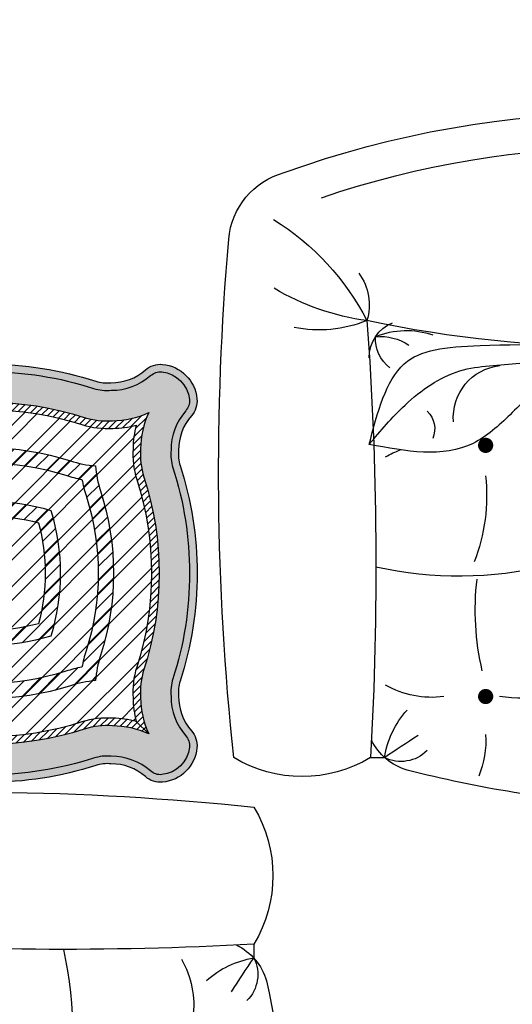
# Model space of a CAD drawing. Units: inches. Extents: x 844 to 2234, y 346 to 1084.
# Tile 23 of 93: x 1105 to 1116, y 710 to 731. Entities that reach past the tile are written whole.
import ezdxf

# ---------------------------------------------------------------- set-up
doc = ezdxf.new("R2010")
doc.units = ezdxf.units.IN
doc.header["$MEASUREMENT"] = 0
doc.layers.add('A-ANNO-DIMS', color=2, linetype='Continuous', lineweight=18)
doc.layers.add('furniture', color=8, linetype='Continuous', lineweight=18)
for name, color, linetype in [('RA-AP-01$0$FURN', 3, 'Continuous'), ('RA-AP-01$0$steel', 193, 'Continuous'), ('RA-AP-01$0$WOOD', 64, 'Continuous')]:
    doc.layers.add(name, color=color, linetype=linetype)
doc.styles.get("Standard").update_dxf_attribs({"font": 'arial.ttf'})
doc.dimstyles.get("Standard").update_dxf_attribs({"dimtxt": 6, "dimasz": 3, "dimexe": 0.18, "dimexo": 0.0625, "dimgap": 0.09, "dimtad": 0, "dimtih": 1, "dimtoh": 1, "dimdec": 1, "dimzin": 0, "dimdsep": 46, "dimlunit": 3, "dimtxsty": 'Standard', "dimblk": 'ARCHTICK', "dimcen": 0.09, "dimadec": 0, "dimazin": 0, "dimtfac": 1, "dimtdec": 1, "dimtofl": 0, "dimtmove": 0, "dimatfit": 3, "dimfxl": 1, "dimtolj": 1, "dimtzin": 0, "dimarcsym": 0})
pattern_1 = [(45, (0, 1.362436106329781), (-0.0088388347648318, 0.0088388347648318), [])]
pattern_2 = [(45, (0, 1.362436106329781), (-0.0044194173824159, 0.0044194173824159), [])]

# ---------------------------------------------------------------- blocks, each defined once
blk = doc.blocks.new('A$C2FCF5309')
at = {"layer": 'RA-AP-01$0$FURN'}
h = blk.add_hatch(dxfattribs=at)
h.set_pattern_fill('ANSI31', color=256, scale=0.1, style=0)
h.set_pattern_definition(pattern_1)
h.paths.add_polyline_path([(5.038683893313746, -5.169250834004607, -0.1583983521602212), (5.038683893312098, -5.373464580902012, 0.0306258898943267), (5.033304057242972, -5.394827569605182, 0.0306258898948892), (5.01194106853941, -5.40020740567441, -0.1028142994996694), (4.878286182323899, -5.414871334512708), (4.863600873530158, -5.43331743520547, 0.1120482678681049), (5.018059823131753, -5.419248541734471, -0.052642197802937), (5.050972078299936, -5.412495590662115, -0.0526421977994963), (5.057725029371615, -5.379583335496025, 0.1583028414702701), (5.057725029372958, -5.163132079409654, -0.052642197806903), (5.050972078299777, -5.130219824239078, -0.0526421977995126), (5.018059823133679, -5.123466873167369, 0.0215995840215353), (4.988903013548211, -5.115372132362452), (4.975007495303644, -5.132826183367946, -0.0289147572844802), (5.011941068537408, -5.142508009226167, 0.0306258898976746), (5.033304057242868, -5.147887845296027, 0.0306258899022411)])
h.paths.add_polyline_path([(4.975007495303645, -5.132826183367946), (4.988903013548211, -5.115372132362452, 0.1362374241599938), (4.801608567045604, -5.12346687316654, -0.0526421978036853), (4.768696311876971, -5.130219824239102, -0.05264219780204), (4.761943360804856, -5.163132079406747, 0.1583028414743723), (4.761943360806116, -5.379583335498449, -0.0526421977955461), (4.768696311877141, -5.412495590662114, -0.0526421978073986), (4.801608567048022, -5.419248541735437, 0.0454484293938888), (4.863600873530158, -5.43331743520547), (4.878286182323899, -5.414871334512708, -0.0546933379798044), (4.80772732164382, -5.40020740567649, 0.030625889903973), (4.786364332934043, -5.394827569605216, 0.0306258898932853), (4.780984496865101, -5.373464580902791, -0.1583983521638281), (4.780984496864308, -5.169250834000963, 0.03062588989692), (4.786364332933943, -5.147887845296004, 0.0306258898946324), (4.807727321637318, -5.142508009226805, -0.1288932573266927)])
h.paths.add_polyline_path([(4.843422214712861, -5.204945727074827, -0.0783685831716868), (4.924134454130224, -5.196727409635105), (4.939146578618322, -5.177870798323143, 0.1012675676854134), (4.827248748758957, -5.188772261120899, 0.1253648873081696), (4.820394258584192, -5.327034652050361), (4.837127701354095, -5.306015906404253, -0.0981593964869636)], flags=17)
h.paths.add_polyline_path([(4.843422214712824, -5.337769687826355, -0.0311091841722656), (4.837127701354095, -5.306015906404253), (4.820394258584193, -5.32703465205036, 0.0247727657431944), (4.827248748758908, -5.353943153780261, 0.0812754385032542), (4.916962478476905, -5.36629034358622), (4.933684093813825, -5.345286454285511, -0.0876255421014372)], flags=17)
h.paths.add_polyline_path([(4.992419641418037, -5.353943153780226, 0.1506053783834298), (4.992419641417933, -5.188772261120954, 0.0485966419124224), (4.939146578618321, -5.177870798323143), (4.924134454130224, -5.196727409635105, -0.0507799419579301), (4.976246175464031, -5.204945727074882, -0.1296645318906876), (4.97624617546411, -5.337769687826316, -0.0415667119298777), (4.933684093813825, -5.345286454285511), (4.916962478476905, -5.36629034358622, 0.0684915676023693)], flags=17)
h = blk.add_hatch(dxfattribs=at)
h.set_pattern_fill('ANSI31', color=256, scale=0.1, style=0)
h.set_pattern_definition(pattern_1)
h.paths.add_polyline_path([(5.038683893313746, -5.169250834004607, -0.1583983521602212), (5.038683893312098, -5.373464580902012, 0.0306258898943267), (5.033304057242972, -5.394827569605182, 0.0306258898948892), (5.01194106853941, -5.40020740567441, -0.1028142994996694), (4.878286182323899, -5.414871334512708), (4.863600873530158, -5.43331743520547, 0.1120482678681049), (5.018059823131753, -5.419248541734471, -0.052642197802937), (5.050972078299936, -5.412495590662115, -0.0526421977994963), (5.057725029371615, -5.379583335496025, 0.1583028414702701), (5.057725029372958, -5.163132079409654, -0.052642197806903), (5.050972078299777, -5.130219824239078, -0.0526421977995126), (5.018059823133679, -5.123466873167369, 0.0215995840215353), (4.988903013548211, -5.115372132362452), (4.975007495303644, -5.132826183367946, -0.0289147572844802), (5.011941068537408, -5.142508009226167, 0.0306258898976746), (5.033304057242868, -5.147887845296027, 0.0306258899022411)])
h.paths.add_polyline_path([(4.975007495303645, -5.132826183367946), (4.988903013548211, -5.115372132362452, 0.1362374241599938), (4.801608567045604, -5.12346687316654, -0.0526421978036853), (4.768696311876971, -5.130219824239102, -0.05264219780204), (4.761943360804856, -5.163132079406747, 0.1583028414743723), (4.761943360806116, -5.379583335498449, -0.0526421977955461), (4.768696311877141, -5.412495590662114, -0.0526421978073986), (4.801608567048022, -5.419248541735437, 0.0454484293938888), (4.863600873530158, -5.43331743520547), (4.878286182323899, -5.414871334512708, -0.0546933379798044), (4.80772732164382, -5.40020740567649, 0.030625889903973), (4.786364332934043, -5.394827569605216, 0.0306258898932853), (4.780984496865101, -5.373464580902791, -0.1583983521638281), (4.780984496864308, -5.169250834000963, 0.03062588989692), (4.786364332933943, -5.147887845296004, 0.0306258898946324), (4.807727321637318, -5.142508009226805, -0.1288932573266927)])
h.paths.add_polyline_path([(4.843422214712861, -5.204945727074827, -0.0783685831716868), (4.924134454130224, -5.196727409635105), (4.939146578618322, -5.177870798323143, 0.1012675676854134), (4.827248748758957, -5.188772261120899, 0.1253648873081696), (4.820394258584192, -5.327034652050361), (4.837127701354095, -5.306015906404253, -0.0981593964869636)], flags=17)
h.paths.add_polyline_path([(4.843422214712824, -5.337769687826355, -0.0311091841722656), (4.837127701354095, -5.306015906404253), (4.820394258584193, -5.32703465205036, 0.0247727657431944), (4.827248748758908, -5.353943153780261, 0.0812754385032542), (4.916962478476905, -5.36629034358622), (4.933684093813825, -5.345286454285511, -0.0876255421014372)], flags=17)
h.paths.add_polyline_path([(4.992419641418037, -5.353943153780226, 0.1506053783834298), (4.992419641417933, -5.188772261120954, 0.0485966419124224), (4.939146578618321, -5.177870798323143), (4.924134454130224, -5.196727409635105, -0.0507799419579301), (4.976246175464031, -5.204945727074882, -0.1296645318906876), (4.97624617546411, -5.337769687826316, -0.0415667119298777), (4.933684093813825, -5.345286454285511), (4.916962478476905, -5.36629034358622, 0.0684915676023693)], flags=17)
at = {"layer": 'RA-AP-01$0$WOOD'}
h = blk.add_hatch(color=256, dxfattribs=at)
edge = h.paths.add_edge_path()
edge.add_arc((4.683001772622394, -5.026441828662609), 0.0299999999999998, 48.77105092035535, 95.25687599427813)
edge.add_arc((4.684834195088484, -5.046357707450686), 0.0499999999998897, 95.25687599443106, 174.7431240064049)
edge.add_arc((4.664918316300367, -5.044525284985046), 0.0300000000000005, 174.7431240062535, 221.2289490796905)
edge.add_arc((4.591236830209155, -5.109094338216345), 0.0679700159630267, -0.5333070513215148, 41.228949079691915, ccw=False)
edge.add_arc((4.609451302807284, -5.114694777173187), 0.0500000000000008, -17.3556839752095, 5.7020707654044145, ccw=False)
edge.add_arc((5.095208119646659, -5.271357707450659), 0.4603971832811796, 162.0683908477609, 197.9316091523306)
edge.add_arc((4.609451302807533, -5.428020637728902), 0.0500000000000006, -5.702070765320514, 17.355683975293914, ccw=False)
edge.add_arc((4.591236830209412, -5.433621076685779), 0.0679700159630261, -41.228949079600625, 0.5333070514128053, ccw=False)
edge.add_arc((4.664918316300727, -5.498190129916959), 0.0299999999999995, 138.7710509204022, 185.256875994324)
edge.add_arc((4.684834195088642, -5.496357707450695), 0.0499999999997451, 185.2568759946742, 264.74312400432)
edge.add_arc((4.683001772622394, -5.516273586238612), 0.03, 264.743124003969, 311.2289490796446)
edge.add_arc((4.747570825853633, -5.589955072329876), 0.0679700159630271, 89.4666929486321, 131.2289490796457, ccw=False)
edge.add_arc((4.753171264810493, -5.57174059973175), 0.0500000000000015, 72.64431602474701, 95.70207076536133, ccw=False)
edge.add_arc((4.909834195088355, -5.085983782892503), 0.4603971832811774, 252.0683908477147, 287.9316091522845)
edge.add_arc((5.06649712536621, -5.57174059973175), 0.0499999999999999, 84.29792923463953, 107.35568397525361, ccw=False)
edge.add_arc((5.072097564323069, -5.589955072329877), 0.0679700159630274, 48.771050920354185, 90.5333070513679, ccw=False)
edge.add_arc((5.136666617554309, -5.516273586238614), 0.0299999999999997, 228.771050920353, 275.2568759942969)
edge.add_arc((5.134834195088338, -5.496357707450417), 0.0499999999999982, 275.2568759942949, 354.7431240057633)
edge.add_arc((5.154750073876535, -5.498190129916372), 0.0299999999999999, 354.7431240057662, 401.2289490796891)
edge.add_arc((5.228431559967749, -5.433621076685074), 0.0679700159630274, 179.4666929486771, 221.2289490796903, ccw=False)
edge.add_arc((5.210217087369615, -5.428020637728227), 0.0499999999999976, 162.6443160247947, 185.7020707654089, ccw=False)
edge.add_arc((4.724460270530244, -5.271357707450757), 0.4603971832811793, 342.0683908477607, 377.9316091523305)
edge.add_arc((5.210217087369368, -5.114694777172509), 0.0500000000000019, 174.2979292346878, 197.355683975302, ccw=False)
edge.add_arc((5.228431559967489, -5.109094338215639), 0.0679700159630279, 138.7710509203993, 180.5333070514128, ccw=False)
edge.add_arc((5.154750073876174, -5.044525284984457), 0.0300000000000001, 318.771050920401, 365.2568759954636)
edge.add_arc((5.13483419508816, -5.046357707450624), 0.0499999999998349, 5.256875995237118, 84.74312400549572)
edge.add_arc((5.136666617554308, -5.026441828662608), 0.0299999999999994, 84.74312400572185, 131.2289490796446)
edge.add_arc((5.072097564323072, -4.952760342571343), 0.0679700159630261, 269.4666929486298, 311.22894907964354, ccw=False)
edge.add_arc((5.066497125366206, -4.97097481516947), 0.0499999999999992, 252.64431602475162, 275.70207076536565, ccw=False)
edge.add_arc((4.909834195088355, -5.456731632008717), 0.4603971832811764, 72.06839084771546, 107.9316091522853)
edge.add_arc((4.753171264810493, -4.970974815169471), 0.0500000000000016, 264.2979292346387, 287.355683975253, ccw=False)
edge.add_arc((4.747570825853633, -4.952760342571346), 0.0679700159630274, 228.7710509203543, 270.5333070513679, ccw=False)
edge = h.paths.add_edge_path(flags=16)
edge.add_arc((4.683001772622395, -5.026441828662608), 0.019999999999999, 48.7710509203555, 95.2568759942793)
edge.add_arc((4.684834195088469, -5.046357707450671), 0.0399999999998731, 95.2568759944489, 174.7431240064248)
edge.add_arc((4.664918316300404, -5.044525284985035), 0.020000000000036, 174.7431240062186, 221.2289490796461)
edge.add_arc((4.591236830209151, -5.109094338216346), 0.0779700159630296, -0.13764630038667747, 41.228949079689585, ccw=False)
edge.add_arc((4.609451302807307, -5.11469477717304), 0.060000000000024, -17.406127045137907, 5.176192161068002, ccw=False)
edge.add_arc((5.09520811964665, -5.271357707450659), 0.4503971832811708, 162.0623235129628, 197.9376764869162)
edge.add_arc((4.609451302807532, -5.428020637728943), 0.0599999999999982, -5.176192160466428, 17.406127046715312, ccw=False)
edge.add_arc((4.591236830209414, -5.433621076685778), 0.0779700159630257, -41.2289490796029, 0.13764630095249686, ccw=False)
edge.add_arc((4.664918316300731, -5.498190129916961), 0.0200000000000047, 138.7710509204103, 185.2568759943212)
edge.add_arc((4.684834195088606, -5.496357707450731), 0.0399999999997066, 185.2568759947174, 264.7431240043665)
edge.add_arc((4.683001772622369, -5.516273586238541), 0.020000000000069, 264.7431240038842, 311.2289490795622)
edge.add_arc((4.747570825853635, -5.589955072329884), 0.0779700159630344, 89.8623536987642, 131.2289490796432, ccw=False)
edge.add_arc((4.753171264810603, -5.571740599731771), 0.0599999999999895, 72.5938729544394, 95.1761921602253, ccw=False)
edge.add_arc((4.909834195088365, -5.085983782892505), 0.4503971832811724, 252.0623235129989, 287.9376764870498)
edge.add_arc((5.066497125366216, -5.571740599731755), 0.0600000000000047, 84.8238078399923, 107.40612704528041, ccw=False)
edge.add_arc((5.072097564322998, -5.589955072329853), 0.077970015963056, 48.771050920303594, 90.13764630126451, ccw=False)
edge.add_arc((5.136666617554307, -5.516273586238622), 0.0199999999999931, 228.771050920344, 275.2568759943037)
edge.add_arc((5.134834195088338, -5.496357707450416), 0.0400000000000004, 275.2568759942928, 354.7431240057607)
edge.add_arc((5.154750073876533, -5.498190129916375), 0.0200000000000037, 354.7431240057783, 401.2289490796939)
edge.add_arc((5.228431559967745, -5.433621076685076), 0.0779700159630239, 179.8623536995147, 221.2289490796908, ccw=False)
edge.add_arc((5.210217087369586, -5.428020637728345), 0.0600000000000054, 162.5938729554486, 185.1761921609759, ccw=False)
edge.add_arc((4.724460270530243, -5.271357707450766), 0.4503971832811826, 342.0623235128896, 377.937676486982)
edge.add_arc((5.210217087369347, -5.114694777172486), 0.0599999999999777, 174.8238078387611, 197.4061270462219, ccw=False)
edge.add_arc((5.228431559967523, -5.109094338215542), 0.0779700159629885, 138.7710509204687, 180.1376463004423, ccw=False)
edge.add_arc((5.154750073876175, -5.044525284984459), 0.0199999999999989, 318.771050920406, 365.2568759954698)
edge.add_arc((5.134834195088138, -5.046357707450646), 0.0399999999998586, 5.256875995208452, 84.74312400546732)
edge.add_arc((5.136666617554292, -5.02644182866256), 0.0199999999999529, 84.74312400577769, 131.2289490797025)
edge.add_arc((5.072097564323069, -4.952760342571338), 0.077970015963032, 269.86235369901414, 311.2289490796421, ccw=False)
edge.add_arc((5.06649712536618, -4.97097481516946), 0.0600000000000007, 252.5938729548277, 275.17619216047467, ccw=False)
edge.add_arc((4.909834195088353, -5.456731632008716), 0.4503971832811739, 72.06232351293887, 107.9376764867365)
edge.add_arc((4.753171264810429, -4.970974815169467), 0.0599999999999991, 264.82380783985815, 287.40612704769893, ccw=False)
edge.add_arc((4.747570825853681, -4.952760342571361), 0.0779700159630467, 228.7710509203206, 270.13764630113724, ccw=False)
h = blk.add_hatch(color=256, dxfattribs=at)
edge = h.paths.add_edge_path()
edge.add_arc((4.683001772622395, -5.026441828662608), 0.019999999999999, 48.7710509203555, 95.2568759942793)
edge.add_arc((4.684834195088469, -5.046357707450671), 0.0399999999998731, 95.2568759944489, 174.7431240064248)
edge.add_arc((4.664918316300404, -5.044525284985035), 0.020000000000036, 174.7431240062186, 221.2289490796461)
edge.add_arc((4.591236830209151, -5.109094338216346), 0.0779700159630296, -0.13764630038667747, 41.228949079689585, ccw=False)
edge.add_arc((4.609451302807307, -5.11469477717304), 0.060000000000024, -17.406127045137907, 5.176192161068002, ccw=False)
edge.add_arc((5.09520811964665, -5.271357707450659), 0.4503971832811708, 162.0623235129628, 197.9376764869162)
edge.add_arc((4.609451302807532, -5.428020637728943), 0.0599999999999982, -5.176192160466428, 17.406127046715312, ccw=False)
edge.add_arc((4.591236830209414, -5.433621076685778), 0.0779700159630257, -41.2289490796029, 0.13764630095249686, ccw=False)
edge.add_arc((4.664918316300731, -5.498190129916961), 0.0200000000000047, 138.7710509204103, 185.2568759943212)
edge.add_arc((4.684834195088606, -5.496357707450731), 0.0399999999997066, 185.2568759947174, 264.7431240043665)
edge.add_arc((4.683001772622369, -5.516273586238541), 0.020000000000069, 264.7431240038842, 311.2289490795622)
edge.add_arc((4.747570825853635, -5.589955072329884), 0.0779700159630344, 89.8623536987642, 131.2289490796432, ccw=False)
edge.add_arc((4.753171264810603, -5.571740599731771), 0.0599999999999895, 72.5938729544394, 95.1761921602253, ccw=False)
edge.add_arc((4.909834195088365, -5.085983782892505), 0.4503971832811724, 252.0623235129989, 287.9376764870498)
edge.add_arc((5.066497125366216, -5.571740599731755), 0.0600000000000047, 84.8238078399923, 107.40612704528041, ccw=False)
edge.add_arc((5.072097564322998, -5.589955072329853), 0.077970015963056, 48.771050920303594, 90.13764630126451, ccw=False)
edge.add_arc((5.136666617554307, -5.516273586238622), 0.0199999999999931, 228.771050920344, 275.2568759943037)
edge.add_arc((5.134834195088338, -5.496357707450416), 0.0400000000000004, 275.2568759942928, 354.7431240057607)
edge.add_arc((5.154750073876533, -5.498190129916375), 0.0200000000000037, 354.7431240057783, 401.2289490796939)
edge.add_arc((5.228431559967745, -5.433621076685076), 0.0779700159630239, 179.8623536995147, 221.2289490796908, ccw=False)
edge.add_arc((5.210217087369586, -5.428020637728345), 0.0600000000000054, 162.5938729554486, 185.1761921609759, ccw=False)
edge.add_arc((4.724460270530243, -5.271357707450766), 0.4503971832811826, 342.0623235128896, 377.937676486982)
edge.add_arc((5.210217087369347, -5.114694777172486), 0.0599999999999777, 174.8238078387611, 197.4061270462219, ccw=False)
edge.add_arc((5.228431559967523, -5.109094338215542), 0.0779700159629885, 138.7710509204687, 180.1376463004423, ccw=False)
edge.add_arc((5.154750073876175, -5.044525284984459), 0.0199999999999989, 318.771050920406, 365.2568759954698)
edge.add_arc((5.134834195088138, -5.046357707450646), 0.0399999999998586, 5.256875995208452, 84.74312400546732)
edge.add_arc((5.136666617554292, -5.02644182866256), 0.0199999999999529, 84.74312400577769, 131.2289490797025)
edge.add_arc((5.072097564323069, -4.952760342571338), 0.077970015963032, 269.86235369901414, 311.2289490796421, ccw=False)
edge.add_arc((5.06649712536618, -4.97097481516946), 0.0600000000000007, 252.5938729548277, 275.17619216047467, ccw=False)
edge.add_arc((4.909834195088353, -5.456731632008716), 0.4503971832811739, 72.06232351293887, 107.9376764867365)
edge.add_arc((4.753171264810429, -4.970974815169467), 0.0599999999999991, 264.82380783985815, 287.40612704769893, ccw=False)
edge.add_arc((4.747570825853681, -4.952760342571361), 0.0779700159630467, 228.7710509203206, 270.13764630113724, ccw=False)
edge = h.paths.add_edge_path(flags=16)
edge.add_arc((4.591236830209151, -5.109094338216348), 0.1179700159630308, 0.7417751874182841, 24.563326950263672, ccw=False)
edge.add_arc((4.609451302807302, -5.114694777173093), 0.100000000000012, -17.52836504564658, 4.087328884225087, ccw=False)
edge.add_arc((5.095208119646651, -5.271357707450657), 0.4103971832811724, 162.0403002448777, 197.9596997550675)
edge.add_arc((4.60945130280753, -5.428020637728918), 0.1000000000000027, -4.087328883827581, 17.528365046291924, ccw=False)
edge.add_arc((4.591236830209414, -5.433621076685779), 0.1179700159630246, 335.43667305041845, 359.2582248129738, ccw=False)
edge.add_arc((4.747570825853596, -5.589955072329891), 0.117970015963042, 90.7417751868461, 114.5633269496104, ccw=False)
edge.add_arc((4.753171264810559, -5.571740599731767), 0.0999999999999976, 72.47163495370341, 94.0873288836737, ccw=False)
edge.add_arc((4.909834195088367, -5.085983782892503), 0.4103971832811735, 252.0403002449999, 287.9596997551833)
edge.add_arc((5.066497125366205, -5.571740599731755), 0.1000000000000057, 85.91267111645209, 107.5283650455624, ccw=False)
edge.add_arc((5.072097564322985, -5.58995507232986), 0.117970015963046, 65.4366730497672, 89.25822481317113, ccw=False)
edge.add_arc((5.22843155996773, -5.433621076684992), 0.1179700159630096, 180.7417751873964, 204.5633269502712, ccw=False)
edge.add_arc((5.210217087369591, -5.428020637728301), 0.0999999999999969, 162.4716349546276, 184.0873288841682, ccw=False)
edge.add_arc((4.724460270530243, -5.271357707450766), 0.4103971832811825, 342.0403002448147, 377.9596997550345)
edge.add_arc((5.210217087369347, -5.114694777172489), 0.0999999999999796, 175.9126711156995, 197.5283650464392, ccw=False)
edge.add_arc((5.228431559967512, -5.109094338215525), 0.1179700159630019, 155.4366730502992, 179.2582248126247, ccw=False)
edge.add_arc((5.072097564323172, -4.952760342571314), 0.1179700159630537, 270.74177518697286, 294.56332694975765, ccw=False)
edge.add_arc((5.066497125366189, -4.970974815169462), 0.1000000000000017, 252.471634954247, 274.0873288838353, ccw=False)
edge.add_arc((4.909834195088353, -5.456731632008716), 0.4103971832811758, 72.04030024486342, 107.9596997549354)
edge.add_arc((4.75317126481046, -4.970974815169467), 0.1000000000000041, 265.91267111635307, 287.5283650466103, ccw=False)
edge.add_arc((4.747570825853629, -4.952760342571342), 0.1179700159630538, 245.43667304992562, 269.2582248131125, ccw=False)
h = blk.add_hatch(dxfattribs=at)
h.set_pattern_fill('ANSI31', color=256, scale=0.05, style=0)
h.set_pattern_definition(pattern_2)
h.paths.add_polyline_path([(5.105336294329346, -5.394854099602528, 0.0940138826956367), (5.100476366643778, -5.435568764288975, 0.0606271852326483), (5.104678567100611, -5.466202079462671, 0.0606271852344644), (5.074045251925975, -5.46199987900586, 0.0940138827021426), (5.033330587236848, -5.466859806692645, -0.1305325492494615), (4.828072633169377, -5.477944178050054), (4.821119726105699, -5.486677669841435, 0.1336226599878005), (5.036379334063467, -5.476383803188216, -0.0945969211935747), (5.073624810952389, -5.471994942692536, -0.1043170707892296), (5.121137550891356, -5.48266106325342, -0.1043170707868944), (5.110471430330457, -5.435148323315565, -0.0945969211952573), (5.114860290825935, -5.397902846425963, 0.1580239521433527), (5.114860290826324, -5.144812568476775, -0.0945969212010491), (5.110471430330247, -5.10756709158498, -0.1043170707844371), (5.121137550890657, -5.060054351648168, -0.104317070786514), (5.073624810952866, -5.070720472208642, -0.0945969211958523), (5.036379334063063, -5.066331611712874, 0.1580239521426795), (4.783289056114906, -5.066331611712465, -0.0945969211985319), (4.746043579224103, -5.070720472208672, -0.1043170707882665), (4.698530839285552, -5.060054351647925, -0.1043170707867205), (4.709196959846443, -5.10756709158571, -0.094596921196788), (4.704808099350826, -5.144812568475902, 0.1580239521433127), (4.704808099350699, -5.397902846425022, -0.094596921197841), (4.709196959846712, -5.435148323315576, -0.1043170707855109), (4.698530839286393, -5.482661063252921, -0.1043170707864168), (4.746043579224162, -5.471994942692571, -0.0945969211977586), (4.783289056114671, -5.476383803188671, 0.0238966994662183), (4.821119726105699, -5.486677669841435), (4.828072633169378, -5.477944178050054, -0.0269814195959459), (4.786337802940177, -5.466859806692736, 0.0940138827039629), (4.745623138250268, -5.461999879005895, 0.0606271852320776), (4.714989823076826, -5.466202079462476, 0.0606271852304618), (4.719192023533341, -5.435568764289856, 0.0940138826917763), (4.714332095848404, -5.394854099604977, -0.1580706864542086), (4.714332095846561, -5.147861315302034, 0.0940138827032017), (4.719192023533127, -5.107146650612438, 0.0606271852329446), (4.714989823076289, -5.076513335438588, 0.0606271852340035), (4.745623138250698, -5.08071553589536, 0.0940138827025969), (4.786337802940015, -5.075855608208526, -0.1580706864508517), (5.033330587237968, -5.075855608208939, 0.0940138827009578), (5.074045251926627, -5.080715535895319, 0.0606271852322557), (5.104678567100159, -5.076513335438697, 0.0606271852308743), (5.100476366643561, -5.107146650611519, 0.0940138827178109), (5.105336294331983, -5.147861315307182, -0.1580706864490946)])
h = blk.add_hatch(dxfattribs=at)
h.set_pattern_fill('ANSI31', color=256, scale=0.05, style=0)
h.set_pattern_definition(pattern_2)
h.paths.add_polyline_path([(5.105336294329346, -5.394854099602528, 0.0940138826956367), (5.100476366643778, -5.435568764288975, 0.0606271852326483), (5.104678567100611, -5.466202079462671, 0.0606271852344644), (5.074045251925975, -5.46199987900586, 0.0940138827021426), (5.033330587236848, -5.466859806692645, -0.1305325492494615), (4.828072633169377, -5.477944178050054), (4.821119726105699, -5.486677669841435, 0.1336226599878005), (5.036379334063467, -5.476383803188216, -0.0945969211935747), (5.073624810952389, -5.471994942692536, -0.1043170707892296), (5.121137550891356, -5.48266106325342, -0.1043170707868944), (5.110471430330457, -5.435148323315565, -0.0945969211952573), (5.114860290825935, -5.397902846425963, 0.1580239521433527), (5.114860290826324, -5.144812568476775, -0.0945969212010491), (5.110471430330247, -5.10756709158498, -0.1043170707844371), (5.121137550890657, -5.060054351648168, -0.104317070786514), (5.073624810952866, -5.070720472208642, -0.0945969211958523), (5.036379334063063, -5.066331611712874, 0.1580239521426795), (4.783289056114906, -5.066331611712465, -0.0945969211985319), (4.746043579224103, -5.070720472208672, -0.1043170707882665), (4.698530839285552, -5.060054351647925, -0.1043170707867205), (4.709196959846443, -5.10756709158571, -0.094596921196788), (4.704808099350826, -5.144812568475902, 0.1580239521433127), (4.704808099350699, -5.397902846425022, -0.094596921197841), (4.709196959846712, -5.435148323315576, -0.1043170707855109), (4.698530839286393, -5.482661063252921, -0.1043170707864168), (4.746043579224162, -5.471994942692571, -0.0945969211977586), (4.783289056114671, -5.476383803188671, 0.0238966994662183), (4.821119726105699, -5.486677669841435), (4.828072633169378, -5.477944178050054, -0.0269814195959459), (4.786337802940177, -5.466859806692736, 0.0940138827039629), (4.745623138250268, -5.461999879005895, 0.0606271852320776), (4.714989823076826, -5.466202079462476, 0.0606271852304618), (4.719192023533341, -5.435568764289856, 0.0940138826917763), (4.714332095848404, -5.394854099604977, -0.1580706864542086), (4.714332095846561, -5.147861315302034, 0.0940138827032017), (4.719192023533127, -5.107146650612438, 0.0606271852329446), (4.714989823076289, -5.076513335438588, 0.0606271852340035), (4.745623138250698, -5.08071553589536, 0.0940138827025969), (4.786337802940015, -5.075855608208526, -0.1580706864508517), (5.033330587237968, -5.075855608208939, 0.0940138827009578), (5.074045251926627, -5.080715535895319, 0.0606271852322557), (5.104678567100159, -5.076513335438697, 0.0606271852308743), (5.100476366643561, -5.107146650611519, 0.0940138827178109), (5.105336294331983, -5.147861315307182, -0.1580706864490946)])
h = blk.add_hatch(dxfattribs=at)
h.set_pattern_fill('ANSI32,_I', color=256, scale=0.1, style=2)
h.set_pattern_definition([(45, (0, 0), (-0.0265165042944955, 0.0265165042944955), []), (45, (0.0176776695, 0), (-0.0265165042944955, 0.0265165042944955), [])])
h.paths.add_polyline_path([(4.843422214712824, -5.337769687826354, 0.1296645318905289), (4.97624617546411, -5.337769687826316, 0.1296645318906876), (4.976246175464032, -5.204945727074882, 0.129664531890418), (4.843422214712861, -5.204945727074827, 0.129664531890765)], flags=0)
h.paths.add_polyline_path([(5.039131224122924, -5.170637849998464, -0.0326520429852175), (5.033304057242868, -5.147887845296027, -0.0326520429894721), (5.010554052537512, -5.142060678415043, 0.1561383235202698), (4.809114337641437, -5.142060678414318, -0.0326520429925972), (4.786364332933944, -5.147887845296004, -0.0326520429914489), (4.780537166052582, -5.170637850002729, 0.1561383235189577), (4.780537166052134, -5.37207756489719, -0.0326520429934175), (4.786364332934042, -5.394827569605215, -0.0326520429823496), (4.809114337634529, -5.400654736484653, 0.156138323524066), (5.010554052535268, -5.400654736486903, -0.032652042992888), (5.033304057242972, -5.394827569605183, -0.0326520429928733), (5.039131224124712, -5.372077564897496, 0.1561383235226786)], flags=0)
h.paths.add_polyline_path([(4.992419641418037, -5.353943153780226, -0.1506053783832862), (4.827248748758909, -5.353943153780261, -0.1506053783835069), (4.827248748758957, -5.188772261120899, -0.1506053783831346), (4.992419641417933, -5.188772261120954, -0.1506053783834298)], flags=0)
h.paths.add_polyline_path([(4.976246175464111, -5.337769687826316, -0.1296645318905298), (4.843422214712824, -5.337769687826354, -0.129664531890765), (4.843422214712862, -5.204945727074827, -0.1296645318904162), (4.976246175464031, -5.204945727074882, -0.1296645318906876)], flags=0)
h.paths.add_polyline_path([(5.105721254232479, -5.149054940982025, -0.0968902512052664), (5.100476366643561, -5.107146650611519, -0.0606271852308743), (5.104678567100159, -5.076513335438697, -0.0606271852322574), (5.074045251926626, -5.080715535895319, -0.0968902512197216), (5.032136961550132, -5.075470648304253, 0.1564657949319774), (4.787531428625239, -5.075470648304682, -0.0968902512150626), (4.745623138250699, -5.08071553589536, -0.060627185234009), (4.714989823076288, -5.076513335438587, -0.0606271852329501), (4.719192023533127, -5.10714665061244, -0.0968902512185585), (4.713947135942331, -5.149054940988458, 0.1564657949285579), (4.713947135940853, -5.393660473908259, -0.0968902512319826), (4.71919202353334, -5.435568764289873, -0.0606271852304288), (4.714989823076825, -5.466202079462476, -0.0606271852320811), (4.745623138250269, -5.461999879005895, -0.0968902512162649), (4.787531428625332, -5.467244766596559, 0.1564657949327057), (5.032136961551311, -5.46724476659659, -0.0968902512153659), (5.074045251925975, -5.46199987900586, -0.0606271852344627), (5.10467856710061, -5.466202079462671, -0.0606271852326483), (5.100476366643777, -5.435568764288975, -0.0968902512258216), (5.105721254235559, -5.393660473909953, 0.1564657949340142)])
h.paths.add_polyline_path([(5.057725029371625, -5.379583335495999, 0.0526421977995391), (5.050972078299936, -5.412495590662114, 0.0526421978029782), (5.018059823131728, -5.419248541734479, -0.1583028414681072), (4.801608567048168, -5.419248541735485, 0.0526421978076402), (4.76869631187714, -5.412495590662113, 0.0526421977956189), (4.761943360806101, -5.379583335498404, -0.1583028414743129), (4.761943360804846, -5.163132079406778, 0.0526421978020944), (4.768696311876972, -5.130219824239101, 0.0526421978033651), (4.80160856704541, -5.123466873166602, -0.1583028414716875), (5.018059823133628, -5.123466873167353, 0.0526421977995944), (5.050972078299776, -5.130219824239078, 0.0526421978070423), (5.057725029372986, -5.163132079409739, -0.1583028414701848)], flags=16)
h.paths.add_polyline_path([(5.038683893312112, -5.373464580901968, 0.0306258898943915), (5.033304057242972, -5.394827569605182, 0.0306258898948892), (5.01194106853941, -5.40020740567441, -0.1583983521587032), (4.807727321643864, -5.400207405676503, 0.0306258899040366), (4.786364332934043, -5.394827569605215, 0.0306258898931986), (4.780984496865119, -5.37346458090285, -0.1583983521638542), (4.7809844968643, -5.169250834000989, 0.0306258898969596), (4.786364332933945, -5.147887845296004, 0.0306258898946195), (4.807727321637311, -5.142508009226808, -0.1583983521623412), (5.011941068537318, -5.142508009226139, 0.030625889897807), (5.033304057242868, -5.147887845296028, 0.0306258899020632), (5.038683893313706, -5.169250834004486, -0.1583983521602835)], flags=0)
for p, q in [((4.714989823076289, -5.076513335438588), (4.698530839285552, -5.060054351647925)), ((4.714989823076289, -5.076513335438588), (4.698530839285552, -5.060054351647925)), ((5.104678567100159, -5.076513335438697), (5.121137550890656, -5.060054351648169)), ((5.104678567100159, -5.076513335438697), (5.121137550890656, -5.060054351648169)), ((5.10467856710061, -5.466202079462671), (5.121137550891355, -5.482661063253419)), ((5.10467856710061, -5.466202079462671), (5.121137550891355, -5.482661063253419))]:
    blk.add_line(p, q, dxfattribs=at)
for points in [[(4.702773858784635, -5.003879368495489, 0.2056608120285223), (4.680253138923443, -4.996568010480312, 0.3614336704708569), (4.635044498118043, -5.041776651286372, 0.2056608120263112), (4.642355856133262, -5.064297371147306, -0.1842662638101064), (4.65920390179375, -5.10972699154053, -0.1009492694051416), (4.657174869772992, -5.129609908955028, 0.1577727036674954), (4.657174869773219, -5.41310550594699, -0.1009492694051416), (4.659203901794006, -5.432988423361486, -0.1842662638101064), (4.64235585613359, -5.478418043754737, 0.2056608120285221), (4.635044498118431, -5.500938763615934, 0.3614336704593693), (4.680253138922529, -5.546147404420826, 0.2056608120364936), (4.702773858784635, -5.538836046405732, -0.1842662638101064), (4.748203479177874, -5.52198800074528, -0.1009492694051415), (4.768086396592371, -5.524017032766053, 0.1577727036674954), (5.051581993584332, -5.524017032766055, -0.1009492694051416), (5.071464910998829, -5.521988000745282, -0.1842662638101064), (5.116894531392067, -5.538836046405734, 0.2056608120286145), (5.13941525125327, -5.546147404420911, 0.3614336704683636), (5.184623892058835, -5.500938763615299, 0.2056608120285223), (5.177312534043641, -5.478418043754112, -0.1842662638101063), (5.160464488383153, -5.432988423360887, -0.1009492694051416), (5.162493520403909, -5.41310550594639, 0.1577727036674954), (5.162493520403684, -5.129609908954428, -0.1009492694051416), (5.160464488382894, -5.109726991539933, -0.1842662638101064), (5.17731253404331, -5.064297371146681, 0.2056608120337072), (5.184623892058415, -5.041776651284888, 0.3614336704623863), (5.139415251253259, -4.99656801048031, 0.2056608120285223), (5.116894531392067, -5.003879368495487, -0.1842662638101064), (5.071464910998829, -5.020727414155937, -0.1009492694051416), (5.051581993584332, -5.018698382135166, 0.1577727036674956), (4.768086396592371, -5.018698382135168, -0.1009492694051416), (4.748203479177874, -5.020727414155941, -0.1842662638101064)], [(4.702773858784635, -5.003879368495489, 0.2056608120285223), (4.680253138923443, -4.996568010480312, 0.3614336704708569), (4.635044498118043, -5.041776651286372, 0.2056608120263112), (4.642355856133262, -5.064297371147306, -0.1842662638101064), (4.65920390179375, -5.10972699154053, -0.1009492694051416), (4.657174869772992, -5.129609908955028, 0.1577727036674954), (4.657174869773219, -5.41310550594699, -0.1009492694051416), (4.659203901794006, -5.432988423361486, -0.1842662638101064), (4.64235585613359, -5.478418043754737, 0.2056608120285221), (4.635044498118431, -5.500938763615934, 0.3614336704593693), (4.680253138922529, -5.546147404420826, 0.2056608120364936), (4.702773858784635, -5.538836046405732, -0.1842662638101064), (4.748203479177874, -5.52198800074528, -0.1009492694051415), (4.768086396592371, -5.524017032766053, 0.1577727036674954), (5.051581993584332, -5.524017032766055, -0.1009492694051416), (5.071464910998829, -5.521988000745282, -0.1842662638101064), (5.116894531392067, -5.538836046405734, 0.2056608120286145), (5.13941525125327, -5.546147404420911, 0.3614336704683636), (5.184623892058835, -5.500938763615299, 0.2056608120285223), (5.177312534043641, -5.478418043754112, -0.1842662638101063), (5.160464488383153, -5.432988423360887, -0.1009492694051416), (5.162493520403909, -5.41310550594639, 0.1577727036674954), (5.162493520403684, -5.129609908954428, -0.1009492694051416), (5.160464488382894, -5.109726991539933, -0.1842662638101064), (5.17731253404331, -5.064297371146681, 0.2056608120337072), (5.184623892058415, -5.041776651284888, 0.3614336704623863), (5.139415251253259, -4.99656801048031, 0.2056608120285223), (5.116894531392067, -5.003879368495487, -0.1842662638101064), (5.071464910998829, -5.020727414155937, -0.1009492694051416), (5.051581993584332, -5.018698382135166, 0.1577727036674956), (4.768086396592371, -5.018698382135168, -0.1009492694051416), (4.748203479177874, -5.020727414155941, -0.1842662638101064)], [(4.696183163397222, -5.011400188551196, 0.2056608120285295), (4.681169350156427, -5.006525949874411, 0.3614336704708588), (4.645002437512154, -5.042692862519237, 0.2056608120262659), (4.649876676188964, -5.057706675759887, -0.182481815856965), (4.669206621172843, -5.109281651732388, -0.0988540857970112), (4.666703803477437, -5.13264334722805, 0.1578269695851905), (4.666703803477144, -5.410072067672365, -0.0988540858013112), (4.6692066211731, -5.433433763168966, -0.1824818158591246), (4.649876676189301, -5.485008739142145, 0.2056608120284717), (4.64500243751253, -5.500022552382944, 0.3614336704593821), (4.681169350155757, -5.536189465026749, 0.2056608120365057), (4.696183163397221, -5.531315226350026, -0.1824818158605826), (4.747758139370833, -5.51198528136619, -0.0988540857951607), (4.771119834866025, -5.514488099061806, 0.1578269695856264), (5.04854855531107, -5.514488099061688, -0.0988540857929677), (5.071910250805761, -5.511985281366138, -0.1824818158609529), (5.123485226779481, -5.531315226350027, 0.2056608120286893), (5.138499040020282, -5.536189465026812, 0.3614336704683556), (5.174665952664737, -5.500022552382323, 0.2056608120284882), (5.169791713987938, -5.485008739141532, -0.1824818158574124), (5.150461769004059, -5.4334337631689, -0.0988540857940221), (5.152964586699289, -5.410072067673927, 0.1578269695858123), (5.1529645866996, -5.132643347228565, -0.0988540858025403), (5.150461769003872, -5.109281651731659, -0.1824818158565006), (5.169791713987599, -5.057706675759273, 0.2056608120337192), (5.174665952664335, -5.042692862518078, 0.3614336704623903), (5.138499040020236, -5.006525949874406, 0.2056608120285323), (5.123485226779481, -5.011400188551195, -0.1824818158594503), (5.071910250806212, -5.03073013353503, -0.09885408579455), (5.048548555311143, -5.028227315839558, 0.1578269695844942), (4.771119834867991, -5.028227315838772, -0.0988540858042156), (4.747758139370745, -5.030730133535067, -0.1824818158603032)], [(4.696183163397222, -5.011400188551196, 0.2056608120285295), (4.681169350156427, -5.006525949874411, 0.3614336704708588), (4.645002437512154, -5.042692862519237, 0.2056608120262659), (4.649876676188964, -5.057706675759887, -0.182481815856965), (4.669206621172843, -5.109281651732388, -0.0988540857970112), (4.666703803477437, -5.13264334722805, 0.1578269695851905), (4.666703803477144, -5.410072067672365, -0.0988540858013112), (4.6692066211731, -5.433433763168966, -0.1824818158591246), (4.649876676189301, -5.485008739142145, 0.2056608120284717), (4.64500243751253, -5.500022552382944, 0.3614336704593821), (4.681169350155757, -5.536189465026749, 0.2056608120365057), (4.696183163397221, -5.531315226350026, -0.1824818158605826), (4.747758139370833, -5.51198528136619, -0.0988540857951607), (4.771119834866025, -5.514488099061806, 0.1578269695856264), (5.04854855531107, -5.514488099061688, -0.0988540857929677), (5.071910250805761, -5.511985281366138, -0.1824818158609529), (5.123485226779481, -5.531315226350027, 0.2056608120286893), (5.138499040020282, -5.536189465026812, 0.3614336704683556), (5.174665952664737, -5.500022552382323, 0.2056608120284882), (5.169791713987938, -5.485008739141532, -0.1824818158574124), (5.150461769004059, -5.4334337631689, -0.0988540857940221), (5.152964586699289, -5.410072067673927, 0.1578269695858123), (5.1529645866996, -5.132643347228565, -0.0988540858025403), (5.150461769003872, -5.109281651731659, -0.1824818158565006), (5.169791713987599, -5.057706675759273, 0.2056608120337192), (5.174665952664335, -5.042692862518078, 0.3614336704623903), (5.138499040020236, -5.006525949874406, 0.2056608120285323), (5.123485226779481, -5.011400188551195, -0.1824818158594503), (5.071910250806212, -5.03073013353503, -0.09885408579455), (5.048548555311143, -5.028227315839558, 0.1578269695844942), (4.771119834867991, -5.028227315838772, -0.0988540858042156), (4.747758139370745, -5.030730133535067, -0.1824818158603032)], [(4.698530839285552, -5.060054351647925, -0.1043170707867612), (4.709196959846444, -5.107567091585729, -0.0945969211969405), (4.704808099350802, -5.144812568475978, 0.1580239521432241), (4.704808099350681, -5.397902846424963, -0.0945969211980322), (4.709196959846711, -5.43514832331559, -0.104317070785482), (4.698530839286393, -5.482661063252921, -0.1043170707864036), (4.746043579224155, -5.471994942692571, -0.094596921197375), (4.78328905611452, -5.476383803188623, 0.1580239521431959), (5.036379334063463, -5.476383803188218, -0.0945969211935888), (5.07362481095239, -5.471994942692536, -0.1043170707892253), (5.121137550891355, -5.482661063253419, -0.1043170707868921), (5.110471430330457, -5.435148323315565, -0.0945969211954828), (5.114860290825962, -5.397902846425878, 0.158023952143358), (5.114860290826295, -5.144812568476682, -0.0945969212007617), (5.110471430330247, -5.107567091584995, -0.1043170707844689), (5.121137550890656, -5.060054351648169, -0.1043170707864946), (5.073624810952874, -5.070720472208642, -0.0945969211956941), (5.036379334063131, -5.066331611712896, 0.1580239521426976), (4.783289056114946, -5.066331611712452, -0.0945969211986379), (4.746043579224103, -5.070720472208672, -0.1043170707882684)], [(4.698530839285552, -5.060054351647925, -0.1043170707867612), (4.709196959846444, -5.107567091585729, -0.0945969211969405), (4.704808099350802, -5.144812568475978, 0.1580239521432241), (4.704808099350681, -5.397902846424963, -0.0945969211980322), (4.709196959846711, -5.43514832331559, -0.104317070785482), (4.698530839286393, -5.482661063252921, -0.1043170707864036), (4.746043579224155, -5.471994942692571, -0.094596921197375), (4.78328905611452, -5.476383803188623, 0.1580239521431959), (5.036379334063463, -5.476383803188218, -0.0945969211935888), (5.07362481095239, -5.471994942692536, -0.1043170707892253), (5.121137550891355, -5.482661063253419, -0.1043170707868921), (5.110471430330457, -5.435148323315565, -0.0945969211954828), (5.114860290825962, -5.397902846425878, 0.158023952143358), (5.114860290826295, -5.144812568476682, -0.0945969212007617), (5.110471430330247, -5.107567091584995, -0.1043170707844689), (5.121137550890656, -5.060054351648169, -0.1043170707864946), (5.073624810952874, -5.070720472208642, -0.0945969211956941), (5.036379334063131, -5.066331611712896, 0.1580239521426976), (4.783289056114946, -5.066331611712452, -0.0945969211986379), (4.746043579224103, -5.070720472208672, -0.1043170707882684)], [(4.714989823076289, -5.076513335438588, -0.0606271852329464), (4.719192023533127, -5.107146650612439, -0.0940138827030756), (4.714332095846578, -5.147861315301983, 0.1580706864542707), (4.714332095848417, -5.394854099605018, -0.0940138826916965), (4.719192023533341, -5.435568764289864, -0.0606271852304462), (4.714989823076826, -5.466202079462476, -0.0606271852320585), (4.745623138250258, -5.461999879005895, -0.0940138827037036), (4.786337802940059, -5.466859806692699, 0.1580706864500221), (5.033330587236783, -5.466859806692666, -0.0940138827023111), (5.074045251925979, -5.46199987900586, -0.060627185234454), (5.10467856710061, -5.466202079462671, -0.0606271852326709), (5.100476366643777, -5.435568764288963, -0.0940138826958686), (5.105336294329379, -5.394854099602421, 0.1580706864489859), (5.105336294331999, -5.147861315307237, -0.0940138827179432), (5.100476366643561, -5.107146650611518, -0.0606271852308726), (5.104678567100159, -5.076513335438697, -0.0606271852322592), (5.074045251926625, -5.080715535895319, -0.094013882701022), (5.03333058723794, -5.075855608208931, 0.1580706864508015), (4.786337802940061, -5.075855608208511, -0.0940138827027143), (4.745623138250695, -5.08071553589536, -0.0606271852339983)], [(4.714989823076289, -5.076513335438588, -0.0606271852329464), (4.719192023533127, -5.107146650612439, -0.0940138827030756), (4.714332095846578, -5.147861315301983, 0.1580706864542707), (4.714332095848417, -5.394854099605018, -0.0940138826916965), (4.719192023533341, -5.435568764289864, -0.0606271852304462), (4.714989823076826, -5.466202079462476, -0.0606271852320585), (4.745623138250258, -5.461999879005895, -0.0940138827037036), (4.786337802940059, -5.466859806692699, 0.1580706864500221), (5.033330587236783, -5.466859806692666, -0.0940138827023111), (5.074045251925979, -5.46199987900586, -0.060627185234454), (5.10467856710061, -5.466202079462671, -0.0606271852326709), (5.100476366643777, -5.435568764288963, -0.0940138826958686), (5.105336294329379, -5.394854099602421, 0.1580706864489859), (5.105336294331999, -5.147861315307237, -0.0940138827179432), (5.100476366643561, -5.107146650611518, -0.0606271852308726), (5.104678567100159, -5.076513335438697, -0.0606271852322592), (5.074045251926625, -5.080715535895319, -0.094013882701022), (5.03333058723794, -5.075855608208931, 0.1580706864508015), (4.786337802940061, -5.075855608208511, -0.0940138827027143), (4.745623138250695, -5.08071553589536, -0.0606271852339983)], [(4.768696311876972, -5.130219824239102, -0.0526421978019087), (4.761943360804882, -5.163132079406667, 0.1583028414744761), (4.761943360806133, -5.379583335498504, -0.0526421977954539), (4.76869631187714, -5.412495590662113, -0.0526421978076619), (4.801608567048181, -5.419248541735488, 0.1583028414681522), (5.0180598231318, -5.419248541734456, -0.0526421978028585), (5.050972078299936, -5.412495590662114, -0.0526421977992923), (5.057725029371576, -5.379583335496149, 0.1583028414703719), (5.057725029372956, -5.163132079409646, -0.0526421978068888), (5.050972078299776, -5.130219824239078, -0.052642197799403), (5.018059823133745, -5.12346687316739, 0.1583028414717216), (4.801608567045482, -5.123466873166579, -0.0526421978034837)], [(4.768696311876972, -5.130219824239102, -0.0526421978019087), (4.761943360804882, -5.163132079406667, 0.1583028414744761), (4.761943360806133, -5.379583335498504, -0.0526421977954539), (4.76869631187714, -5.412495590662113, -0.0526421978076619), (4.801608567048181, -5.419248541735488, 0.1583028414681522), (5.0180598231318, -5.419248541734456, -0.0526421978028585), (5.050972078299936, -5.412495590662114, -0.0526421977992923), (5.057725029371576, -5.379583335496149, 0.1583028414703719), (5.057725029372956, -5.163132079409646, -0.0526421978068888), (5.050972078299776, -5.130219824239078, -0.052642197799403), (5.018059823133745, -5.12346687316739, 0.1583028414717216), (4.801608567045482, -5.123466873166579, -0.0526421978034837)], [(4.786364332933944, -5.147887845296004, -0.0306258898969254), (4.780984496864308, -5.169250834000966, 0.1583983521638412), (4.780984496865107, -5.373464580902811, -0.0306258898932568), (4.786364332934043, -5.394827569605216, -0.0306258899041339), (4.80772732164393, -5.400207405676526, 0.1583983521586416), (5.011941068539401, -5.400207405674413, -0.0306258898949021), (5.033304057242972, -5.394827569605182, -0.0306258898943513), (5.038683893312104, -5.373464580901996, 0.1583983521602784), (5.038683893313717, -5.16925083400452, -0.0306258899021139), (5.033304057242868, -5.147887845296027, -0.030625889897777), (5.011941068537338, -5.142508009226145, 0.1583983521624288), (4.807727321637224, -5.142508009226835, -0.0306258898944937)], [(4.786364332933944, -5.147887845296004, -0.0306258898969254), (4.780984496864308, -5.169250834000966, 0.1583983521638412), (4.780984496865107, -5.373464580902811, -0.0306258898932568), (4.786364332934043, -5.394827569605216, -0.0306258899041339), (4.80772732164393, -5.400207405676526, 0.1583983521586416), (5.011941068539401, -5.400207405674413, -0.0306258898949021), (5.033304057242972, -5.394827569605182, -0.0306258898943513), (5.038683893312104, -5.373464580901996, 0.1583983521602784), (5.038683893313717, -5.16925083400452, -0.0306258899021139), (5.033304057242868, -5.147887845296027, -0.030625889897777), (5.011941068537338, -5.142508009226145, 0.1583983521624288), (4.807727321637224, -5.142508009226835, -0.0306258898944937)], [(4.827248748758957, -5.1887722611209, 0.1506053783835061), (4.827248748758908, -5.353943153780261, 0.150605378383287), (4.992419641418037, -5.353943153780226, 0.1506053783834298), (4.992419641417933, -5.188772261120954, 0.1506053783831346)], [(4.827248748758957, -5.1887722611209, 0.1506053783835061), (4.827248748758908, -5.353943153780261, 0.150605378383287), (4.992419641418037, -5.353943153780226, 0.1506053783834298), (4.992419641417933, -5.188772261120954, 0.1506053783831346)], [(4.843422214712861, -5.204945727074827, 0.1296645318907659), (4.843422214712824, -5.337769687826355, 0.1296645318905299), (4.976246175464111, -5.337769687826316, 0.1296645318906876), (4.976246175464032, -5.204945727074882, 0.129664531890418)], [(4.843422214712861, -5.204945727074827, 0.1296645318907659), (4.843422214712824, -5.337769687826355, 0.1296645318905299), (4.976246175464111, -5.337769687826316, 0.1296645318906876), (4.976246175464032, -5.204945727074882, 0.129664531890418)]]:
    blk.add_lwpolyline(points, format="xyb", close=True, dxfattribs=at)
blk = doc.blocks.new('A$C7EE91E48')
at = {"layer": 'RA-AP-01$0$FURN'}
blk.add_line((9.775453681024517, -8.916612252413607), (9.757112325609974, -8.91661225241228), dxfattribs=at)
for centre, radius, start, end in [((9.387879261544771, -10.44238280163197), 1.579145581857318, 77.59199468308728, 96.58839125635443), ((9.865453681024029, -9.0661122524033), 0.1744999999876311, 58.95177800404677, 121.0482219959531), ((9.706394910853488, -8.972574909806593), 0.0753785023123622, 25.87456190605585, 73.98335472300344), ((9.735181781955493, -8.959417410432842), 0.0479292786975047, 62.80708685435548, 135.4025460716553), ((9.125600268712216, -8.003664990327692), 1.11020813118073, 301.9328608597714, 304.6664773187981), ((9.636732167011939, -8.897645467382876), 0.1218651776285568, 318.0375529564433, 351.0462320954125), ((14.24233490628227, -9.167687782925107), 4.473931917517753, 176.7828902523826, 184.1477233631118), ((6.42249118116022, -9.291612252417751), 3.552808610866049, 355.0473312316413, 6.058872375658039), ((9.695285873781074, -9.11718462924615), 0.1214118203512435, 60.14190744855965, 97.69166328915595), ((9.65905457432348, -9.665283690153952), 0.5100538472773755, 77.61824893593078, 103.3122231353938)]:
    blk.add_arc(centre, radius, start, end, dxfattribs=at)
blk = doc.blocks.new('A$C7F4351E2')
at = {"layer": 'RA-AP-01$0$FURN'}
blk.add_line((8.352559572600457, -8.927748273106442), (8.35255957259913, -8.909406917691898), dxfattribs=at)
at = {"layer": 'RA-AP-01$0$FURN', "const_width": 0.01}
for points in [[(8.437812509519787, -8.776330465863198, -1), (8.427812509519786, -8.776330465863225, -1)], [(8.758197489244363, -8.776330465862753, 1), (8.768197489244365, -8.776330465862753, 1)]]:
    blk.add_lwpolyline(points, format="xyb", close=True, dxfattribs=at)
at = {"layer": 'RA-AP-01$0$FURN'}
for centre, radius, start, end in [((7.88981694267423, -8.595845114309485), 1.310286319972027, 340.1192502251003, 19.8807497748998), ((7.929864357850293, -8.595845114309483), 1.224941341589781, 341.1257460634955, 18.87425393650447), ((10.52713941284929, -8.595845114309466), 1.634931324962266, 168.1200364254424, 191.8799635745573), ((9.82633505008426, -8.495018853398156), 1.539060359583382, 183.7562265681581, 194.4661216781742), ((8.73287643248165, -8.721914330412496), 0.3023568492824586, 162.411939214449, 186.9055174488332), ((9.101231010340802, -8.811349166405407), 0.5100538472773755, 166.6877768646062, 192.3817510640693), ((8.799643412436344, -8.749969313933361), 0.0689028341546707, 265.5384273543114, 353.5804828909086), ((8.374918524725835, -8.897369025622035), 0.1212957045587361, 86.26852490575668, 112.6624160255178), ((8.697701155637269, -9.019222100351342), 0.2442261434243043, 84.00760748083387, 111.0982929264395), ((8.546954810732721, -8.438295803862992), 0.3517162425384579, 256.8325429434429, 276.5875103323888), ((8.553131949433, -8.847580465862999), 0.1214118203512435, 172.308336710844, 209.8580925514404), ((8.785133372574222, -8.874256642962408), 0.0310151388417235, 42.62105484496073, 114.2239681486109), ((8.395364730619693, -8.88747637403742), 0.0479292786975047, 134.5974539283447, 207.1929131456445), ((8.810121490949696, -8.880582651403534), 0.1042084262671507, 337.1307060672183, 19.51716812828453), ((7.439612310514541, -8.277894860794142), 1.11020813118073, 325.333522681202, 328.0671391402286), ((8.408522229993444, -8.858689502935416), 0.0753785023123622, 196.0166452769965, 244.1254380939442), ((8.333592787569726, -8.789026759093863), 0.1218651776285568, 278.9537679045875, 311.9624470435567), ((8.838100984994732, -8.914867270759315), 0.0683206773889159, 354.781604957363, 33.32701385065517), ((8.642878049331348, -8.847580465862874), 0.1214118203512435, 330.1419074487191, 340.3913536181062), ((8.903279781571525, -8.873311572516016), 0.0478550828899777, 217.3166170761785, 273.424704368466), ((8.878389979098333, -8.879487683384612), 0.05, 270.0000000009465, 337.4173275753961), ((8.603635103111959, -13.39462949836419), 4.473931917517753, 85.85227663688822, 93.21710974761734), ((8.50205957259015, -9.017748273105955), 0.1744999999876311, 148.9517780040469, 211.0482219959533), ((9.084915705374858, -8.995650093654042), 0.1698955038956699, 158.1487616198804, 191.122156864055), ((8.947672844970796, -8.999855035972608), 0.0704710051510922, 53.58735038429053, 106.8661365794674), ((8.77247054904813, -9.233146364837223), 0.3382138395168437, 31.74362916573515, 62.76966729059727), ((9.2484631175852, -8.88899749098148), 0.3241573581843151, 187.6973649013944, 210.7014325157311), ((9.025650106946005, -9.014702826981493), 0.1, 274.9526687683584, 344.500505399143), ((8.727559572604601, -5.574785773242145), 3.552808610866049, 263.941127624342, 274.9526687683587)]:
    blk.add_arc(centre, radius, start, end, dxfattribs=at)
for points, knots in [([(8.764421239581775, -8.929562504990262), (8.755250524728652, -8.881106864374377), (8.74196437992213, -8.810906376383404), (8.80604948961138, -8.740469753734786), (8.847474678848357, -8.701097198289744), (8.897142214037096, -8.58322730303861), (8.897091569728207, -8.784804210134517), (8.88612504526093, -8.897825917224484), (8.806539053396843, -8.9185794820093), (8.764421239581775, -8.92956250499026)], [0, 0, 0, 0, 0.1367586589314792, 0.1981301758052368, 0.2677729570689282, 0.3281194902553322, 0.4737578340741565, 0.5765194025309516, 0.6920332287422236, 0.6920332287422236, 0.6920332287422236, 0.6920332287422236]), ([(8.764421239581775, -8.92956250499026), (8.782204778269502, -8.914603263160053), (8.821592007255505, -8.881471326160916), (8.86917941606436, -8.814322636989944), (8.867818990542759, -8.729338202119969), (8.881231406199264, -8.676770566934765), (8.888101821971249, -8.649843164808122)], [0, 0, 0, 0, 0.070018540671015, 0.1550780383534498, 0.2344491945777043, 0.3178048737568289, 0.3178048737568289, 0.3178048737568289, 0.3178048737568289])]:
    blk.add_open_spline(points, degree=3, knots=knots, dxfattribs=at)
blk = doc.blocks.new('A$C5D2F253E')
at = {"layer": 'RA-AP-01$0$steel', "xscale": -1}
blk.add_blockref('A$C2FCF5309', (6.339960502260055, 7.248884637679282), dxfattribs=at)
at = {"layer": 'RA-AP-01$0$WOOD', "xscale": -1, "rotation": 180}
for name, p in [('A$C7EE91E48', (-8.833013809079146, -7.288751725733902)), ('A$C7F4351E2', (-7.164808785335935, -7.45332973198748))]:
    blk.add_blockref(name, p, dxfattribs=at)
blk = doc.blocks.new('_ArchTick')
at = {"color": 0, "linetype": 'ByBlock', "const_width": 0.15}
blk.add_lwpolyline([(-0.5, -0.5), (0.5, 0.5)], dxfattribs=at)
blk = doc.blocks.new('*D144')
at = {"layer": 'A-ANNO-DIMS', "color": 0, "lineweight": -2, "transparency": 16777216}
for p, q in [((1096.615948, 439.3732739999999), (1096.615948, 1074.743301)), ((1096.615948, 1074.563301), (1102.481950728513, 1074.563301)), ((1143.115948, 1074.563301), (1137.249945271487, 1074.563301)), ((1143.115948, 492.373274), (1143.115948, 1074.743301))]:
    blk.add_line(p, q, dxfattribs=at)
at = {"layer": 'Defpoints', "color": 0, "transparency": 16777216}
for p in [(1143.115948, 1074.563301), (1143.115948, 492.3107739999999), (1096.615948, 439.3107739999999)]:
    blk.add_point(p, dxfattribs=at)
at = {"layer": 'A-ANNO-DIMS', "color": 0, "lineweight": -2, "transparency": 16777216, "xscale": 3, "yscale": 3, "zscale": 3, "rotation": 180}
blk.add_blockref('_ArchTick', (1096.615948, 1074.563301), dxfattribs=at)
at = {"layer": 'A-ANNO-DIMS', "color": 0, "lineweight": -2, "transparency": 16777216, "xscale": 3, "yscale": 3, "zscale": 3}
blk.add_blockref('_ArchTick', (1143.115948, 1074.563301), dxfattribs=at)
at = {"layer": 'A-ANNO-DIMS', "color": 0, "transparency": 16777216, "insert": (1119.865948, 1074.563301), "char_height": 6, "attachment_point": 5}
blk.add_mtext('\\A1;3\'-10 1/2"', dxfattribs=at)

msp = doc.modelspace()

# ---------------------------------------------------------------- block references
at = {"layer": 'furniture', "xscale": 15.94108302203742, "yscale": 15.94108302203742, "zscale": 15.94108302203742, "rotation": 90}
msp.add_blockref('A$C5D2F253E', (1136.147844094663, 696.2584716700112), dxfattribs=at)

# ---------------------------------------------------------------- dimensions: what is measured, and where the dimension line sits
at = {"layer": 'A-ANNO-DIMS'}
dim = msp.add_linear_dim(base=(1143.115948, 1074.563301), p1=(1096.615948, 439.3107739999999), p2=(1143.115948, 492.3107739999999), dimstyle='Standard', override={"dimdec": 1, "dimlfac": 1, "dimrnd": 0, "dimzin": 1, "dimdsep": 46, "dimlunit": 4, "dimfrac": 2}, dxfattribs=at)
dim.commit()
dim.dimension.update_dxf_attribs({"geometry": '*D144', "text_midpoint": (1119.865948, 1074.563301)})

doc.saveas('drawing.dxf')
